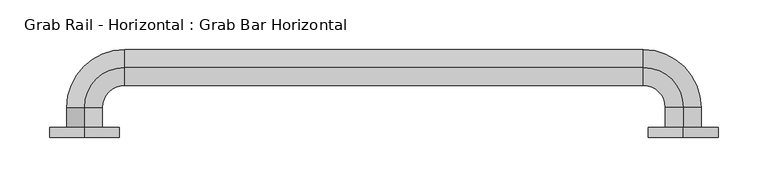
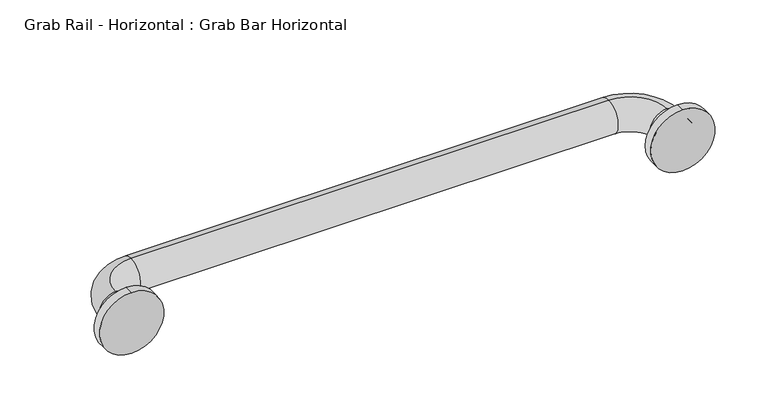
"""IFC4 building model written with IfcOpenShell, lengths in millimetres: flow terminal geometry, Grab Rail - Horizontal : Grab Bar Horizontal."""

from ifc_helpers import new_model, si_unit, point, frame, frame_2d, origin, place, context, project, spatial, circle_curve, ellipse_curve, trimmed, segment, composite_curve, outline, extrude, source, transform, mapped, element, save
from ifc_brep_helpers import plane_surface, cylinder_surface, revolved_surface, advanced_brep


def grab_rail_horizontal_grab_bar_horizontal_f73a8c0c(model_context):
    return source(origin(), model_context, "Body", "SolidModel", [
        extrude(outline(composite_curve([segment(trimmed(circle_curve(frame_2d((680.0, -555.7956665)), 35.0), [point((645.0, -555.7956665))], [point((715.0, -555.7956665))], False, "CARTESIAN"), True, "CONTINUOUS"), segment(trimmed(circle_curve(frame_2d((680.0, -555.7956665)), 35.0), [point((715.0, -555.7956665))], [point((645.0, -555.7956665))], False, "CARTESIAN"), True, "CONTINUOUS")], self_intersect=False)), frame((0.0, 0.0, 0.0), z_axis=(0.0, 1.0, 0.0), x_axis=(0.0, 0.0, 1.0)), (0.0, 0.0, 1.0), 10.0),
        extrude(outline(composite_curve([segment(trimmed(circle_curve(frame_2d((680.0, -1155.7956665)), 35.0), [point((645.0, -1155.7956665))], [point((715.0, -1155.7956665))], False, "CARTESIAN"), True, "CONTINUOUS"), segment(trimmed(circle_curve(frame_2d((680.0, -1155.7956665)), 35.0), [point((715.0, -1155.7956665))], [point((645.0, -1155.7956665))], False, "CARTESIAN"), True, "CONTINUOUS")], self_intersect=False)), frame((0.0, 0.0, 0.0), z_axis=(0.0, 1.0, 0.0), x_axis=(0.0, 0.0, 1.0)), (0.0, 0.0, 1.0), 10.0),
        advanced_brep(
        [(-555.7956665, 10.0, 698.0), (-555.7956665, 10.0, 662.0), (-555.7956665, 30.0, 698.0), (-555.7956665, 30.0, 662.0), (-595.7956665, 70.0, 662.0), (-595.7956665, 70.0, 698.0), (-1115.7956665, 70.0, 698.0), (-1115.7956665, 70.0, 662.0), (-1155.7956665, 30.0, 662.0), (-1155.7956665, 30.0, 698.0), (-1155.7956665, 10.0, 698.0), (-1155.7956665, 10.0, 662.0)],
        [
            (0, 1, circle_curve(frame((-555.7956665, 10.0, 680.0), z_axis=(0.0, -1.0, 0.0), x_axis=(0.0, 0.0, -1.0)), 18.0)),
            (1, 0, circle_curve(frame((-555.7956665, 10.0, 680.0), z_axis=(0.0, -1.0, 0.0), x_axis=(0.0, 0.0, -1.0)), 18.0)),
            (0, 2),
            (2, 3, circle_curve(frame((-555.7956665, 30.0, 680.0), z_axis=(0.0, -1.0, 0.0), x_axis=(0.0, 0.0, -1.0)), 18.0)),
            (3, 1),
            (3, 2, circle_curve(frame((-555.7956665, 30.0, 680.0), z_axis=(0.0, -1.0, 0.0), x_axis=(0.0, 0.0, -1.0)), 18.0)),
            (4, 3, circle_curve(frame((-595.7956665, 30.0, 662.0), z_axis=(0.0, 0.0, -1.0), x_axis=(1.0, 0.0, 0.0)), 40.0)),
            (2, 5, circle_curve(frame((-595.7956665, 30.0, 698.0), z_axis=(0.0, 0.0, 1.0), x_axis=(1.0, 0.0, 0.0)), 40.0)),
            (5, 4, circle_curve(frame((-595.7956665, 70.0, 680.0), z_axis=(1.0, 0.0, 0.0), x_axis=(0.0, 0.0, -1.0)), 18.0)),
            (4, 5, circle_curve(frame((-595.7956665, 70.0, 680.0), z_axis=(1.0, 0.0, 0.0), x_axis=(0.0, 0.0, -1.0)), 18.0)),
            (5, 6),
            (6, 7, circle_curve(frame((-1115.7956665, 70.0, 680.0), z_axis=(1.0, 0.0, 0.0), x_axis=(0.0, 0.0, -1.0)), 18.0)),
            (7, 4),
            (7, 6, circle_curve(frame((-1115.7956665, 70.0, 680.0), z_axis=(1.0, 0.0, 0.0), x_axis=(0.0, 0.0, -1.0)), 18.0)),
            (8, 7, circle_curve(frame((-1115.7956665, 30.0, 662.0), z_axis=(0.0, 0.0, -1.0), x_axis=(0.0, 1.0, 0.0)), 40.0)),
            (6, 9, circle_curve(frame((-1115.7956665, 30.0, 698.0), z_axis=(0.0, 0.0, 1.0), x_axis=(0.0, 1.0, 0.0)), 40.0)),
            (9, 8, circle_curve(frame((-1155.7956665, 30.0, 680.0), z_axis=(0.0, 1.0, 0.0), x_axis=(0.0, 0.0, -1.0)), 18.0)),
            (8, 9, circle_curve(frame((-1155.7956665, 30.0, 680.0), z_axis=(0.0, 1.0, 0.0), x_axis=(0.0, 0.0, -1.0)), 18.0)),
            (10, 11, circle_curve(frame((-1155.7956665, 10.0, 680.0), z_axis=(0.0, -1.0, 0.0), x_axis=(0.0, 0.0, -1.0)), 18.0)),
            (11, 10, circle_curve(frame((-1155.7956665, 10.0, 680.0), z_axis=(0.0, -1.0, 0.0), x_axis=(0.0, 0.0, -1.0)), 18.0)),
            (9, 10),
            (11, 8),
        ],
        [
            plane_surface(frame((-555.7956665, 10.0, 680.0), z_axis=(0.0, -1.0, 0.0), x_axis=(0.0, 0.0, 1.0))),
            cylinder_surface(frame((-555.7956665, 10.0, 680.0), z_axis=(0.0, -1.0, 0.0), x_axis=(0.0, 0.0, -1.0)), 18.0),
            revolved_surface(trimmed(ellipse_curve(frame((-555.7956665, 30.0, 680.0), z_axis=(0.0, -1.0, 0.0), x_axis=(0.0, 0.0, -1.0)), 18.0, 18.0), [point((-555.7956665, 30.0, 698.0))], [point((-555.7956665, 30.0, 662.0))], True, "CARTESIAN"), (-595.7956665, 30.0, 680.0), (0.0, 0.0, 1.0)),
            revolved_surface(trimmed(ellipse_curve(frame((-555.7956665, 30.0, 680.0), z_axis=(0.0, -1.0, 0.0), x_axis=(0.0, 0.0, -1.0)), 18.0, 18.0), [point((-555.7956665, 30.0, 662.0))], [point((-555.7956665, 30.0, 698.0))], True, "CARTESIAN"), (-595.7956665, 30.0, 680.0), (0.0, 0.0, 1.0)),
            cylinder_surface(frame((-595.7956665, 70.0, 680.0), z_axis=(1.0, 0.0, 0.0), x_axis=(0.0, 0.0, -1.0)), 18.0),
            revolved_surface(trimmed(ellipse_curve(frame((-1115.7956665, 70.0, 680.0), z_axis=(1.0, 0.0, 0.0), x_axis=(0.0, 0.0, -1.0)), 18.0, 18.0), [point((-1115.7956665, 70.0, 698.0))], [point((-1115.7956665, 70.0, 662.0))], True, "CARTESIAN"), (-1115.7956665, 30.0, 680.0), (0.0, 0.0, 1.0)),
            revolved_surface(trimmed(ellipse_curve(frame((-1115.7956665, 70.0, 680.0), z_axis=(1.0, 0.0, 0.0), x_axis=(0.0, 0.0, -1.0)), 18.0, 18.0), [point((-1115.7956665, 70.0, 662.0))], [point((-1115.7956665, 70.0, 698.0))], True, "CARTESIAN"), (-1115.7956665, 30.0, 680.0), (0.0, 0.0, 1.0)),
            plane_surface(frame((-1155.7956665, 10.0, 680.0), z_axis=(0.0, -1.0, 0.0), x_axis=(0.0, 0.0, 1.0))),
            cylinder_surface(frame((-1155.7956665, 30.0, 680.0), z_axis=(0.0, 1.0, 0.0), x_axis=(0.0, 0.0, -1.0)), 18.0),
        ],
        [
            (0, [[1, 2]]),
            (1, [[-1, 3, 4, 5]]),
            (1, [[-2, -5, 6, -3]]),
            (2, [[7, -4, 8, 9]]),
            (3, [[-8, -6, -7, 10]]),
            (4, [[-9, 11, 12, 13]]),
            (4, [[-10, -13, 14, -11]]),
            (5, [[15, -12, 16, 17]]),
            (6, [[-16, -14, -15, 18]]),
            (7, [[19, 20]]),
            (8, [[-17, 21, -20, 22]]),
            (8, [[-18, -22, -19, -21]]),
        ],
    ),
    ])


if __name__ == "__main__":
    model = new_model("IFC4")
    model_context = context("Model", 3, world=origin())
    ifc_project = project(units=[si_unit("LENGTHUNIT", "METRE", prefix="MILLI")], contexts=[model_context])
    site = spatial("IfcSite", under=ifc_project)
    building = spatial("IfcBuilding", under=site)
    placement = place(None, origin())
    grab_rail_horizontal_grab_bar_horizontal_shape = grab_rail_horizontal_grab_bar_horizontal_f73a8c0c(model_context)
    element("IfcFlowTerminal", 1, ObjectType="Grab Rail - Horizontal : Grab Bar Horizontal", at=placement, inside=building, context=model_context, shape_type="MappedRepresentation", body=[
        mapped(grab_rail_horizontal_grab_bar_horizontal_shape, transform((0.0, 0.0, 0.0), x_axis=(1.0, 0.0, 0.0), y_axis=(0.0, 1.0, 0.0), z_axis=(0.0, 0.0, 1.0))),
    ])
    save(model, "model.ifc")

# Revit data of these elements
# Type "Grab Rail - Horizontal : Grab Bar Horizontal"
#   Keynote = "N13"
#   Material SanitaryWare [instance default] = Metal - White powder coated
#   Default Elevation = 0
#   Assembly Code = ""
# Element 1 (IfcFlowTerminal, "Grab Rail - Horizontal : Grab Bar Horizontal")
#   Materials on its faces: "Metal - White powder coated"
# Materials
#   "Metal - White powder coated": colour RGB 249 249 249, transparency 0
